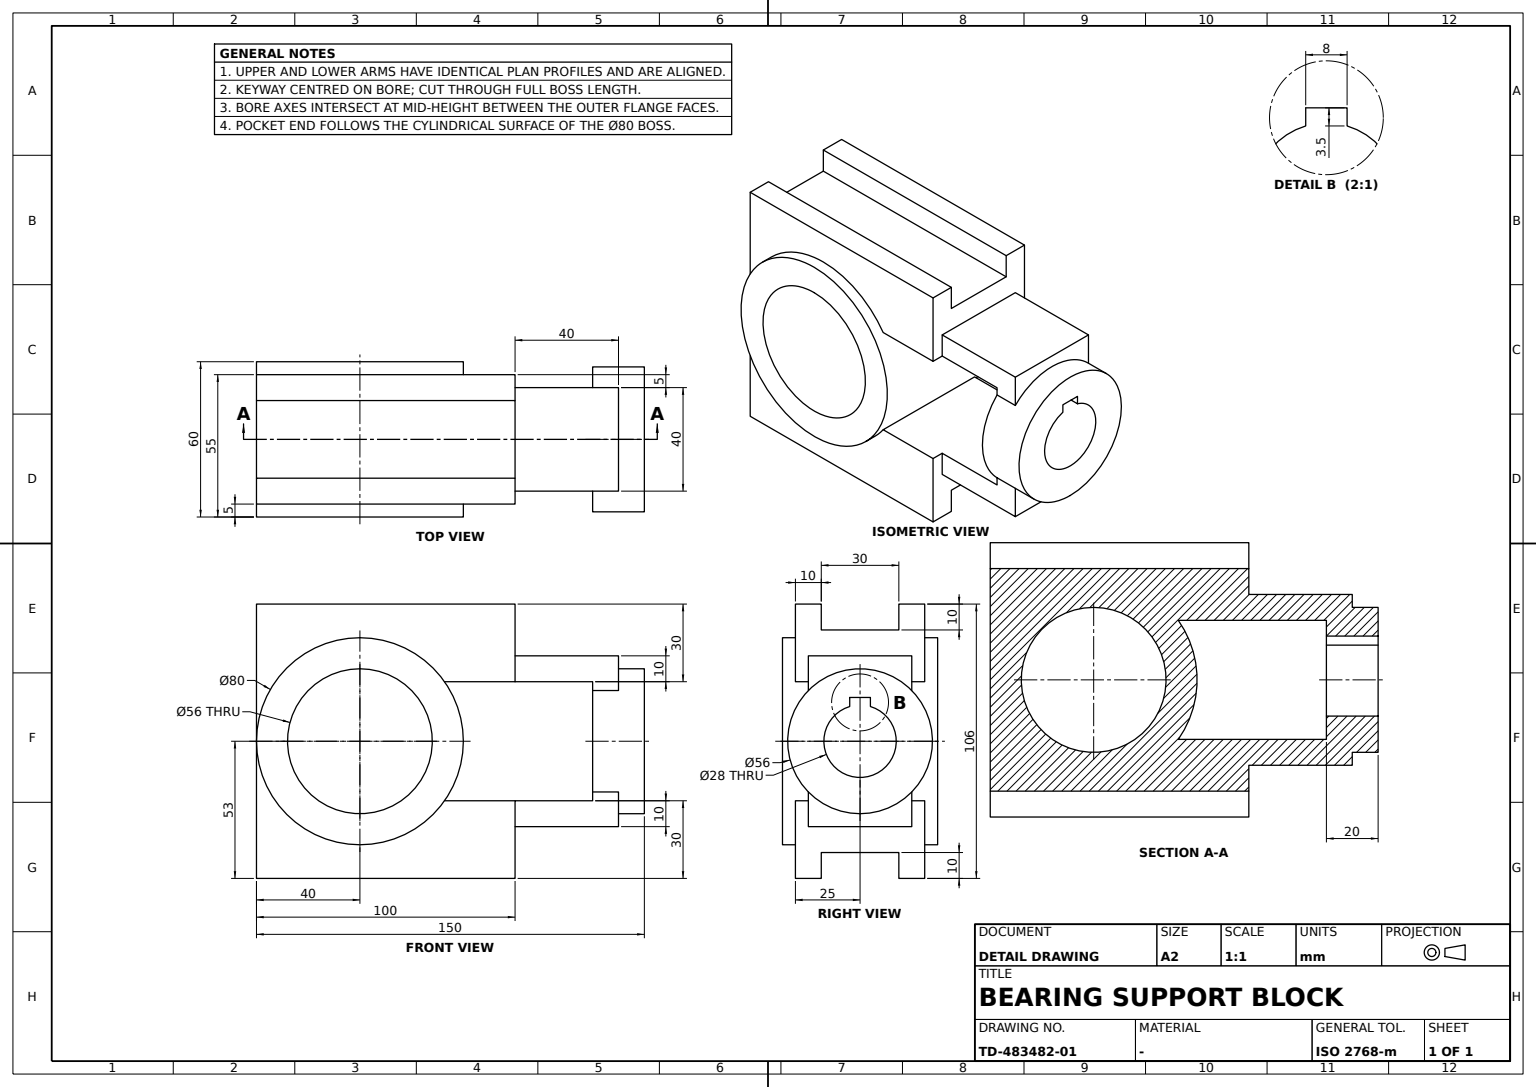
CATIA V5 part; units mm, degrees
sketch "Sketch1" plane through (0, 0, 0) normal (0, 1, 0) x (-1, 0, 0)
  line L0 (0, 0) -> (0, 106)
  line L1 (0, 106) -> (-100, 106)
  line L2 (-100, 106) -> (-100, 76)
  line L3 (-100, 76) -> (-70, 76)
  line L4 (-70, 76) -> (-70, 30)
  line L5 (-70, 30) -> (-100, 30)
  point P0 (-100, 30)
  line L6 (-100, 30) -> (-100, 0)
  point P1 (-100, 0)
  line L7 (-100, 0) -> (0, 0)
  dimension "length L0" = 106
  dimension "length L1" = 100
  dimension "length L2" = 30
  dimension "length L6" = 30
  dimension "length L5" = 30
  constraint vertical L0 y-axis
  constraint vertical L2 y-axis
  constraint vertical L4 y-axis
  constraint vertical L6 y-axis
  constraint horizontal L1 x-axis
  constraint horizontal L3 x-axis
  constraint horizontal L5 x-axis
  constraint horizontal L7 x-axis
  constraint coincidence P0 L2
  constraint coincidence P1 x-axis
extrude "Pad1" add sketch "Sketch1" along normal mid plane 50
sketch "Sketch2" plane through (0, 25, 0) normal (0, 1, 0) x (-1, 0, 0)
  circle A0 centre (-40, 53) radius 40
  point P0 (-40, 53)
  line L0 (0, 106) -> (-100, 106) construction
  line L1 (0, 0) -> (0, 106) construction
  dimension "radius A0" = 40
  dimension "distance P0 L0" = 53
  constraint tangency A0 L1
extrude "Pad2" add sketch "Sketch2" along normal blind 5 and the other way blind 55
sketch "Sketch3" plane through (43.591, 30, 79.0116) normal (0, 1, 0) x (1, 0, 0)
  point P0 (-3.591, 26.0116)
  circle A0 centre (-3.591, 26.0116) radius 40 construction
  constraint concentricity A0 P0
hole "Hole1" at (40, 30, 53) direction (0, -1, 0) diameter 56 end up to next
sketch "Sketch4" plane through (100, 0, 0) normal (1, 0, 0) x (0, 1, 0)
  line L0 (-15, 106) -> (15, 106)
  line L1 (15, 106) -> (15, 96)
  line L2 (15, 96) -> (-15, 96)
  line L3 (-15, 96) -> (-15, 106)
  line L4 (-25, 106) -> (25, 106) construction
  point P0 (0, 70.6091)
  line L5 (-15, 0) -> (15, 0)
  line L6 (15, 0) -> (15, 10)
  line L7 (15, 10) -> (-15, 10)
  line L8 (-15, 10) -> (-15, 0)
  dimension "length L0" = 30
  dimension "length L1" = 10
  dimension "length L6" = 10
  dimension "length L7" = 30
  constraint horizontal L0 x-axis
  constraint horizontal L2 x-axis
  constraint vertical L1 y-axis
  constraint vertical L3 y-axis
  constraint coincidence L0 L4
  constraint coincidence P0 y-axis
extrude "Pocket1" cut sketch "Sketch4" against normal up to next
sketch "Sketch5" plane through (100, 0, 0) normal (1, 0, 0) x (0, 1, 0)
  line L0 (-20, 86) -> (20, 86)
  line L1 (20, 86) -> (20, 76)
  line L2 (20, 76) -> (-20, 76)
  line L3 (-20, 76) -> (-20, 86)
  line L4 (-25, 76) -> (25, 76) construction
  line L5 (25, 106) -> (25, 76) construction
  line L6 (-20, 20) -> (20, 20)
  line L7 (20, 20) -> (20, 30)
  line L8 (20, 30) -> (-20, 30)
  line L9 (-20, 30) -> (-20, 20)
  dimension "length L1" = 10
  dimension "length L0" = 40
  dimension "distance L1 L5" = 5
  constraint horizontal L0 x-axis
  constraint horizontal L2 x-axis
  constraint vertical L1 y-axis
  constraint vertical L3 y-axis
  constraint coincidence L2 L4
extrude "Pad3" add sketch "Sketch5" along normal blind 40
sketch "Sketch6" plane through (0, 20, 0) normal (0, 1, 0) x (-1, 0, 0)
  line L0 (-140, 76) -> (-130, 76)
  line L1 (-130, 76) -> (-130, 30)
  line L2 (-130, 30) -> (-140, 30)
  line L3 (-140, 30) -> (-140, 76)
  line L4 (-100, 30) -> (-140, 30) construction
  line L5 (-140, 20) -> (-140, 30) construction
  line L6 (-100, 76) -> (-140, 76) construction
  dimension "length L0" = 10
  constraint horizontal L0 x-axis
  constraint horizontal L2 x-axis
  constraint vertical L1 y-axis
  constraint vertical L3 y-axis
  constraint coincidence L2 L4
  constraint coincidence L3 L5
  constraint coincidence L0 L6
extrude "Pad4" add sketch "Sketch6" against normal blind 40
sketch "Sketch7" plane through (140, 0, 0) normal (1, 0, 0) x (0, 1, 0)
  circle A0 centre (0, 53) radius 28
  point P0 (0, 53)
  line L0 (20, 30) -> (20, 20) construction
  dimension "radius A0" = 28
  dimension "distance P0 L0" = 20
  dimension "D3" = 53
extrude "Pad5" add sketch "Sketch7" along normal mid plane 20
sketch "Sketch8" plane through (150, 0, 0) normal (1, 0, 0) x (0, 1, 0)
  arc A0 (-4, 66.4164) -> (4, 66.4164) centre (0, 53) ccw
  point P0 (0, 53)
  line L0 (-25, 0) -> (25, 0) construction
  line L1 (-4, 69.9164) -> (4, 69.9164)
  line L2 (4, 69.9164) -> (4, 66.4164)
  line L3 (-4, 66.4164) -> (-4, 69.9164)
  point P1 (4, 66.4164)
  point P2 (-4, 66.4164)
  point P3 (0, 63.2501)
  point P4 (4, 66.4164)
  point P5 (-4, 66.4164)
  line L4 (0, 67.3792) -> (0, 64.6686) construction
  point P6 (0, 66.0239)
  dimension "radius A0" = 14
  dimension "distance P0 L0" = 53
  dimension "length L1" = 8
  dimension "length L2" = 3.5
  dimension "distance L2 L4" = 4
  constraint coincidence P0 y-axis
  constraint coincidence P3 y-axis
  constraint coincidence L2 P4
  constraint coincidence L3 P5
  constraint coincidence P6 y-axis
  constraint coincidence P2 P5
  constraint coincidence P1 P4
  constraint horizontal L1 x-axis
  constraint vertical L2 y-axis
  constraint vertical L3 y-axis
  constraint vertical L4 y-axis
  constraint midpoint L4 P6
extrude "Pocket2" cut sketch "Sketch8" against normal blind 20
properties part number "catia 28"
